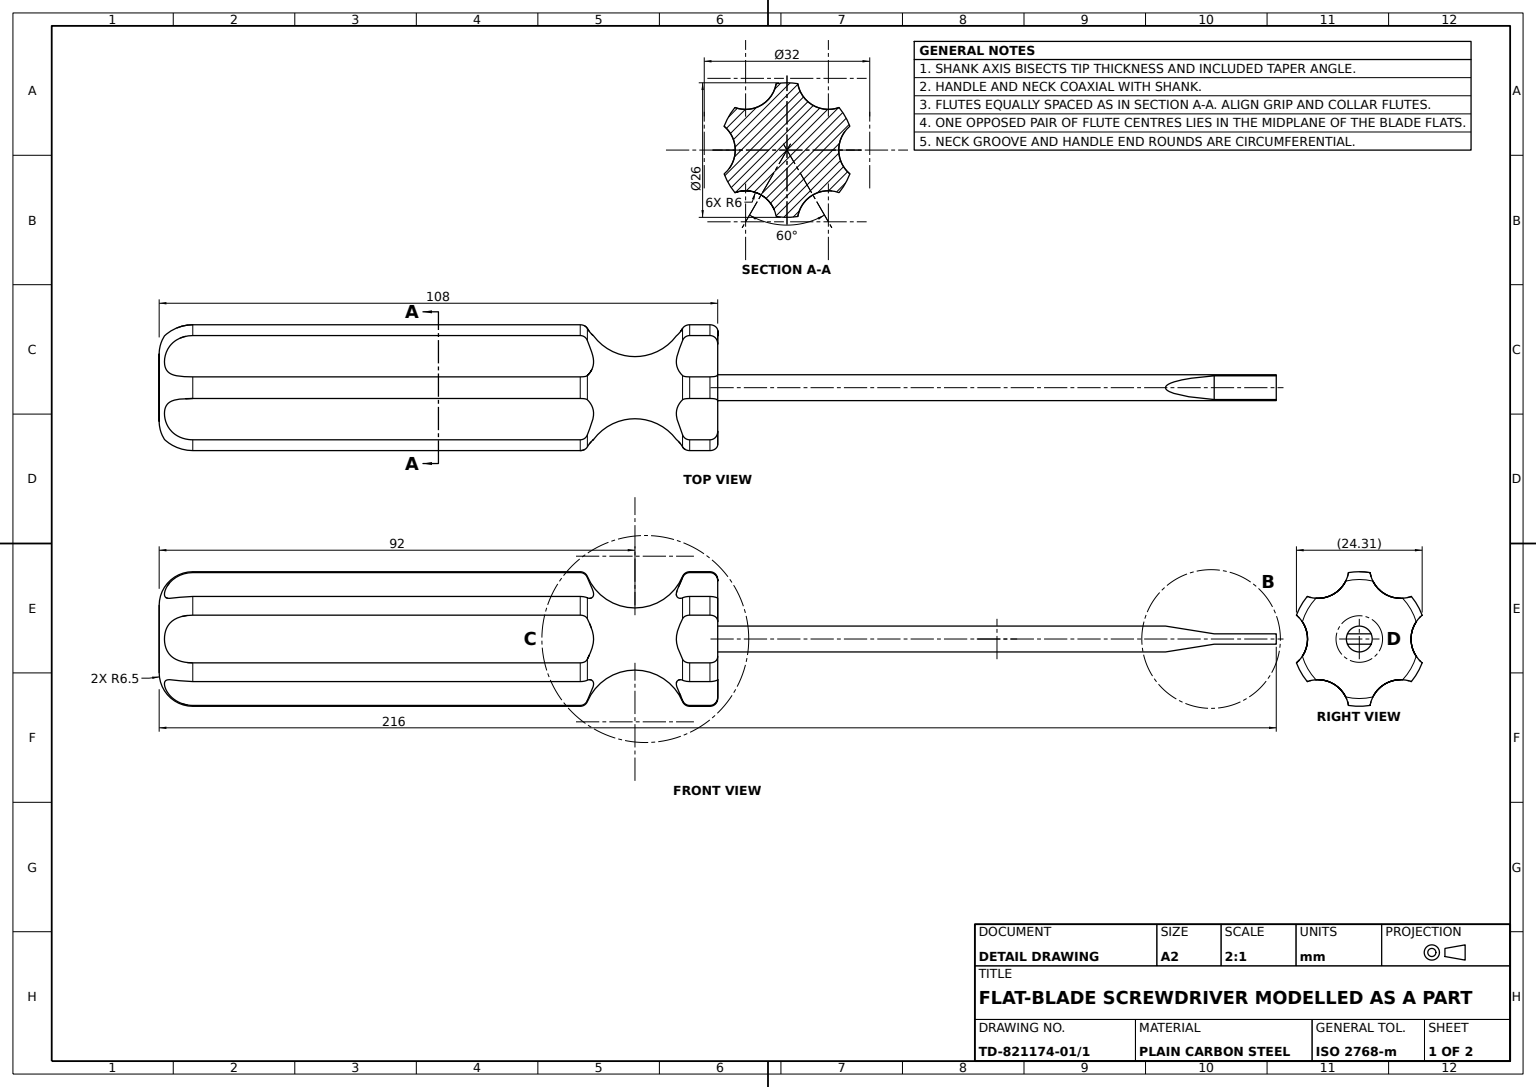
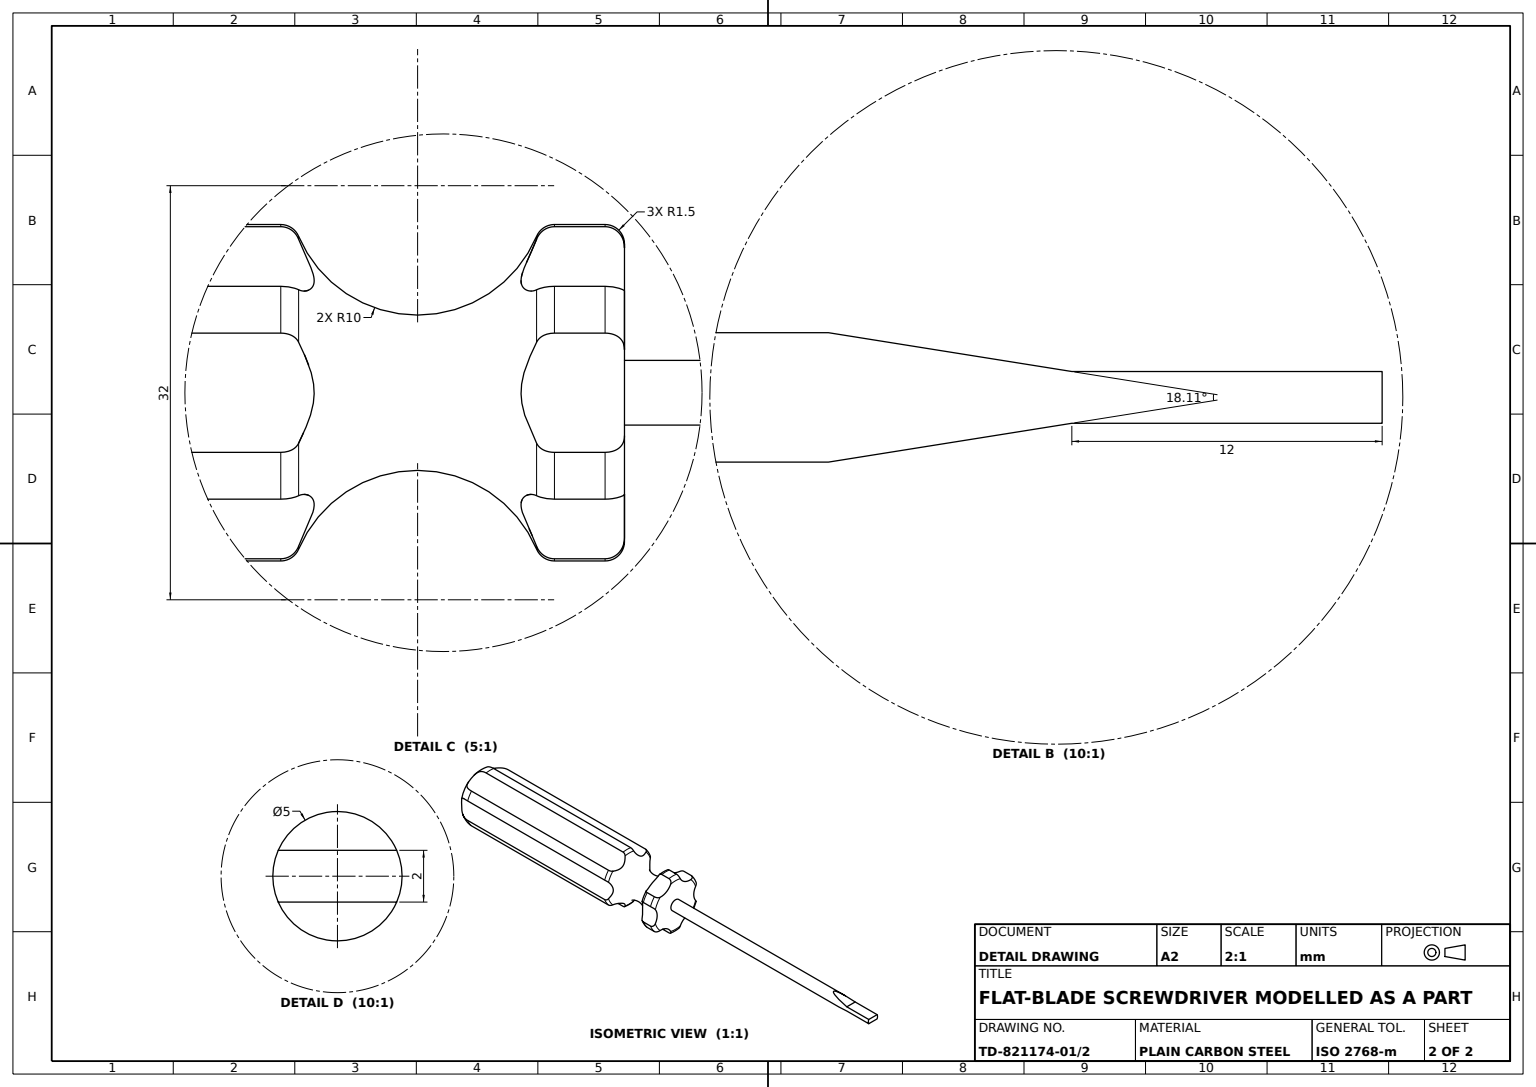
from build123d import *

# Parameters (mm, degrees)
HANDLE_END_FILLET_R6_5_R     = 6.5
COLLAR_FLUTE_CUT_8_6_DEPTH   = 8.6
NECK_GROOVE_SKETCH_R         = 10
BLADE_SHAFT_PROFILE_SKETCH_W = 160
BLADE_SHAFT_PROFILE_SKETCH_H = 2.5
GROOVE_EDGE_FILLET_R1_5_A_R  = 1.5
GROOVE_EDGE_FILLET_R1_5_B_R  = 1.5
GROOVE_EDGE_FILLET_R1_5_C_R  = 1.5
HANDLE_FLUTES_CUT_DEPTH      = 164.039872916
HANDLE_FLUTES_CUT_DEPTH_BACK = 164.039872916
BLADE_TIP_FLAT_CUT_DEPTH     = 217.732033726


with BuildPart() as part:
    # Handle Profile Sketch → Handle Body Revolve (revolve)
    with BuildSketch(Plane(origin=(0, 0, 0), x_dir=(0, 0, -1), z_dir=(1, 0, 0)), mode=Mode.PRIVATE) as handle_body_revolve_sk:
        with BuildLine():
            Line((0, 0), (0, 13))
            Line((0, 13), (101.5, 13))
            Line((101.5, 13), (106.5, 13))
            ThreePointArc((106.5, 13), (107.560660172, 12.560660172), (108, 11.5))
            Line((108, 11.5), (108, 0))
            Line((108, 0), (0, 0))
        make_face()
    revolve(handle_body_revolve_sk.sketch.rotate(Axis((0, 0, -108), (0, 0, 1)), 90), axis=Axis((0, 0, -108), (0, 0, 1)))

    # Handle End Fillet R6.5
    handle_end_fillet_r6_5_edges = [part.edges().sort_by_distance(p)[0] for p in [
        (13, 0, 0),
    ]]
    fillet(handle_end_fillet_r6_5_edges, radius=HANDLE_END_FILLET_R6_5_R)

    # Flute Lobe Profile Sketch → Collar Flute Cut 8.6 (cut)
    with BuildSketch(Plane(origin=(0, 0, -108), x_dir=(-1, 0, 0), z_dir=(0, 0, -1))):
        with BuildLine():
            ThreePointArc((-4.607123391, 12.15625), (0, 10), (4.607123391, 12.15625))
            ThreePointArc((4.607123391, 12.15625), (0, 13), (-4.607123391, 12.15625))
        make_face()
        with BuildLine():
            ThreePointArc((8.224059619, 10.068010895), (8.660254038, 5), (12.83118301, 2.088239105))
            ThreePointArc((12.83118301, 2.088239105), (11.258330249, 6.5), (8.224059619, 10.068010895))
        make_face()
        with BuildLine():
            ThreePointArc((12.83118301, -2.088239105), (8.660254038, -5), (8.224059619, -10.068010895))
            ThreePointArc((8.224059619, -10.068010895), (11.258330249, -6.5), (12.83118301, -2.088239105))
        make_face()
        with BuildLine():
            ThreePointArc((4.607123391, -12.15625), (0, -10), (-4.607123391, -12.15625))
            ThreePointArc((-4.607123391, -12.15625), (0, -13), (4.607123391, -12.15625))
        make_face()
        with BuildLine():
            ThreePointArc((-8.224059619, -10.068010895), (-8.660254038, -5), (-12.83118301, -2.088239105))
            ThreePointArc((-12.83118301, -2.088239105), (-11.258330249, -6.5), (-8.224059619, -10.068010895))
        make_face()
        with BuildLine():
            ThreePointArc((-12.83118301, 2.088239105), (-8.660254038, 5), (-8.224059619, 10.068010895))
            ThreePointArc((-8.224059619, 10.068010895), (-11.258330249, 6.5), (-12.83118301, 2.088239105))
        make_face()
    extrude(amount=-COLLAR_FLUTE_CUT_8_6_DEPTH, mode=Mode.SUBTRACT)

    # Neck Groove Sketch → Neck Groove Cut (revolve, cut)
    with BuildSketch(Plane(origin=(0, 0, 0), x_dir=(0, 0, -1), z_dir=(1, 0, 0)), mode=Mode.PRIVATE) as neck_groove_cut_sk:
        with Locations((92, 16)):
            Circle(NECK_GROOVE_SKETCH_R)
    revolve(neck_groove_cut_sk.sketch.rotate(Axis((0, 0, 0), (0, 0, -1)), 99.243684827), axis=Axis((0, 0, 0), (0, 0, -1)), mode=Mode.SUBTRACT)

    # Blade Shaft Profile Sketch → Blade Shaft Ø5 Revolve (revolve)
    with BuildSketch(Plane(origin=(0, 0, 0), x_dir=(0, 0, -1), z_dir=(1, 0, 0)), mode=Mode.PRIVATE) as blade_shaft_5_revolve_sk:
        with Locations((136, 1.25)):
            Rectangle(BLADE_SHAFT_PROFILE_SKETCH_W, BLADE_SHAFT_PROFILE_SKETCH_H)
    revolve(blade_shaft_5_revolve_sk.sketch.rotate(Axis((0, 0, -56), (0, 0, -1)), 90), axis=Axis((0, 0, -56), (0, 0, -1)))

    # Groove Edge Fillet R1.5 A
    groove_edge_fillet_r1_5_a_edges = [part.edges().sort_by_distance(p)[0] for p in [
        (-1.047525863, -12.957727022, -82.460607986),
    ]]
    fillet(groove_edge_fillet_r1_5_a_edges, radius=GROOVE_EDGE_FILLET_R1_5_A_R)

    # Groove Edge Fillet R1.5 B
    groove_edge_fillet_r1_5_b_edges = [part.edges().sort_by_distance(p)[0] for p in [
        (13, 0, -101.539392014),
        (6.5, -11.258330249, -101.539392014),
    ]]
    fillet(groove_edge_fillet_r1_5_b_edges, radius=GROOVE_EDGE_FILLET_R1_5_B_R)

    # Groove Edge Fillet R1.5 C
    groove_edge_fillet_r1_5_c_edges = [part.edges().sort_by_distance(p)[0] for p in [
        (6.5, 11.258330249, -101.539392014),
        (-6.5, 11.258330249, -101.539392014),
        (-13, 0, -101.539392014),
        (-6.5, -11.258330249, -101.539392014),
    ]]
    fillet(groove_edge_fillet_r1_5_c_edges, radius=GROOVE_EDGE_FILLET_R1_5_C_R)

    # Handle Flute Sketch → Handle Flutes Cut (cut, two sides: drawn at the far end of the back side and taken through both)
    with BuildSketch(Plane.XY.offset(-54).offset(-HANDLE_FLUTES_CUT_DEPTH_BACK)):
        with BuildLine():
            ThreePointArc((8.224059619, 10.068010895), (8.660254038, 5), (12.83118301, 2.088239105))
            ThreePointArc((12.83118301, 2.088239105), (11.258330249, 6.5), (8.224059619, 10.068010895))
        make_face()
        with BuildLine():
            ThreePointArc((12.83118301, -2.088239105), (8.660254038, -5), (8.224059619, -10.068010895))
            ThreePointArc((8.224059619, -10.068010895), (11.258330249, -6.5), (12.83118301, -2.088239105))
        make_face()
        with BuildLine():
            ThreePointArc((4.607123391, -12.15625), (0, -10), (-4.607123391, -12.15625))
            ThreePointArc((-4.607123391, -12.15625), (0, -13), (4.607123391, -12.15625))
        make_face()
        with BuildLine():
            ThreePointArc((-8.224059619, -10.068010895), (-8.660254038, -5), (-12.83118301, -2.088239105))
            ThreePointArc((-12.83118301, -2.088239105), (-11.258330249, -6.5), (-8.224059619, -10.068010895))
        make_face()
        with BuildLine():
            ThreePointArc((-12.83118301, 2.088239105), (-8.660254038, 5), (-8.224059619, 10.068010895))
            ThreePointArc((-8.224059619, 10.068010895), (-11.258330249, 6.5), (-12.83118301, 2.088239105))
        make_face()
        with BuildLine():
            ThreePointArc((-4.607123391, 12.15625), (0, 10), (4.607123391, 12.15625))
            ThreePointArc((4.607123391, 12.15625), (0, 13), (-4.607123391, 12.15625))
        make_face()
    extrude(amount=HANDLE_FLUTES_CUT_DEPTH + HANDLE_FLUTES_CUT_DEPTH_BACK, mode=Mode.SUBTRACT)

    # Blade Tip Flat Sketch → Blade Tip Flat Cut (cut, symmetric)
    with BuildSketch(Plane(origin=(0, 0, 0), x_dir=(1, 0, 0), z_dir=(0, 1, 0))):
        Polygon((-1, 216), (-1, 204), (-2.5, 194.588144223), (-2.5, 216), align=None)
    blade_tip_flat_cut = extrude(amount=BLADE_TIP_FLAT_CUT_DEPTH, both=True, mode=Mode.SUBTRACT)

    # Blade Tip Flat Mirror: Blade Tip Flat Cut across plane
    add(blade_tip_flat_cut.mirror(Plane(origin=(0, 0, 0), x_dir=(0, 0, 1), z_dir=(1, 0, 0))), mode=Mode.SUBTRACT)


solid = part.part
